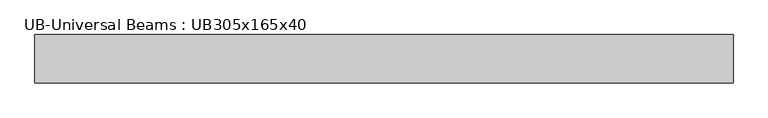
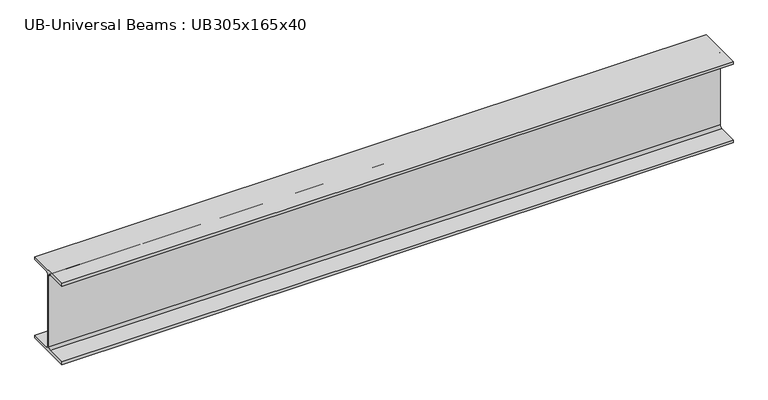
"""IFC4 building model written with IfcOpenShell, lengths in millimetres: beam geometry, UB-Universal Beams : UB305x165x40."""

from ifc_helpers import new_model, si_unit, point, frame, frame_2d, origin, place, context, project, spatial, polyline, circle_curve, trimmed, segment, composite_curve, outline, extrude, source, transform, mapped, element, save


def ub_universal_beams_ub305x165x40_49db3f17(model_context):
    return source(origin(), model_context, "Body", "SweptSolid", [
        extrude(outline(composite_curve([segment(polyline([(82.5, -141.5), (82.5, -151.7), (-82.5, -151.7), (-82.5, -141.5), (-11.9, -141.5)]), True, "CONTINUOUS"), segment(trimmed(circle_curve(frame_2d((-11.9, -132.6)), 8.9), [point((-11.9, -141.5))], [point((-3.0, -132.6))], True, "CARTESIAN"), True, "CONTINUOUS"), segment(polyline([(-3.0, -132.6), (-3.0, 132.6)]), True, "CONTINUOUS"), segment(trimmed(circle_curve(frame_2d((-11.9, 132.6)), 8.9), [point((-3.0, 132.6))], [point((-11.9, 141.5))], True, "CARTESIAN"), True, "CONTINUOUS"), segment(polyline([(-11.9, 141.5), (-82.5, 141.5), (-82.5, 151.7), (82.5, 151.7), (82.5, 141.5), (11.9, 141.5)]), True, "CONTINUOUS"), segment(trimmed(circle_curve(frame_2d((11.9, 132.6)), 8.9), [point((11.9, 141.5))], [point((3.0, 132.6))], True, "CARTESIAN"), True, "CONTINUOUS"), segment(polyline([(3.0, 132.6), (3.0, -132.6)]), True, "CONTINUOUS"), segment(trimmed(circle_curve(frame_2d((11.9, -132.6)), 8.9), [point((3.0, -132.6))], [point((11.9, -141.5))], True, "CARTESIAN"), True, "CONTINUOUS"), segment(polyline([(11.9, -141.5), (82.5, -141.5)]), True, "CONTINUOUS")], self_intersect=False)), frame((-1108.85, 0.0, 0.0), z_axis=(1.0, 0.0, 0.0), x_axis=(0.0, 1.0, 0.0)), (0.0, 0.0, 1.0), 2372.4),
    ])


if __name__ == "__main__":
    model = new_model("IFC4")
    model_context = context("Model", 3, world=origin())
    ifc_project = project(units=[si_unit("LENGTHUNIT", "METRE", prefix="MILLI")], contexts=[model_context])
    site = spatial("IfcSite", under=ifc_project)
    building = spatial("IfcBuilding", under=site)
    placement = place(None, origin())
    ub_universal_beams_ub305x165x40_shape = ub_universal_beams_ub305x165x40_49db3f17(model_context)
    element("IfcBeam", 1, ObjectType="UB-Universal Beams : UB305x165x40", at=placement, inside=building, context=model_context, shape_type="MappedRepresentation", body=[
        mapped(ub_universal_beams_ub305x165x40_shape, transform((0.0, 0.0, 0.0), x_axis=(1.0, 0.0, 0.0), y_axis=(0.0, 1.0, 0.0), z_axis=(0.0, 0.0, 1.0))),
    ])
    save(model, "model.ifc")

# Revit data of these elements
# Type "UB-Universal Beams : UB305x165x40"
#   Section Name Key = "UB305X165X40"
#   Width = 16.5 cm
#   Web Thickness = 0.6 cm
#   Web Fillet = 0.89 cm
#   Warping Constant = 164000.0 cm⁶
#   Torsional Moment of Inertia = 14.70 cm⁴
#   Section Area = 51.3 cm²
#   Plastic Modulus weak axis = 142.0 cm³
#   Plastic Modulus strong axis = 623.0 cm³
#   Nominal Weight = 40.2999 kgf/m
#   Moment of Inertia weak axis = 764.00 cm⁴
#   Moment of Inertia strong axis = 8503.00 cm⁴
#   Height = 30.34 cm
#   Flange Thickness = 1.02 cm
#   Elastic Modulus weak axis = 92.6 cm³
#   Elastic Modulus strong axis = 560.0 cm³
#   Centroid Vertical = 15.17 cm
#   Centroid Horizontal = 8.25 cm
#   Bolt Spacing = 9.0 cm
#   Length [instance default] = 1500 mm
#   Structural Material [instance default] = Metal - Steel 43-275
#   Type Comments = ""
#   Assembly Code = ""
# Element 1 (IfcBeam, "UB-Universal Beams : UB305x165x40")
#   Materials on its faces: "Metal - Steel 43-275"
# Materials
#   "Metal - Steel 43-275": class "Metal", colour RGB 247 247 247, transparency 0, Cost = 0
